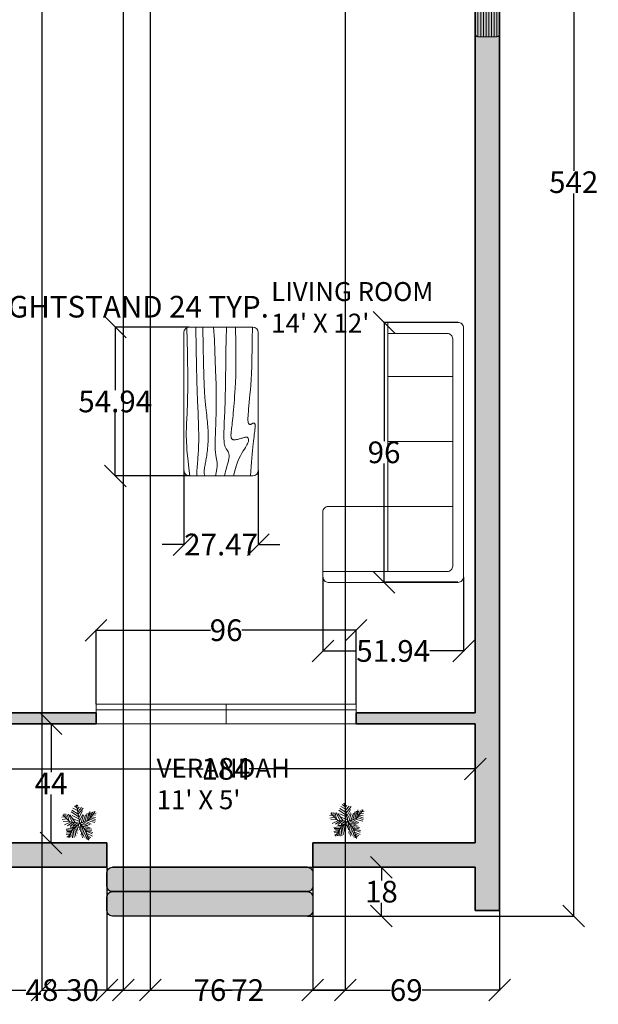
# Model space of a CAD drawing. Units: inches. Extents: x -8 to 447, y -560 to 47.
# Tile 2 of 5: x 201 to 415, y -560 to -196. Entities that reach past the tile are written whole.
import ezdxf

# ---------------------------------------------------------------- set-up
doc = ezdxf.new("R2010")
doc.units = ezdxf.units.IN
doc.header["$MEASUREMENT"] = 0
for name, color, linetype, lineweight in [('A-ANNO-DIMS', 2, 'Continuous', 18), ('A-AREA-IDEN', 7, 'Continuous', 18), ('A-FLOR-PATT', 251, 'Continuous', 13), ('A-FLOR-STRS', 7, 'Continuous', 25), ('A-FURN', 8, 'Continuous', 18), ('A-WALL', 7, 'Continuous', 35), ('A-WALL-PATT', 251, 'Continuous', 13), ('DOOR', 40, 'Continuous', 18), ('PLANTS', 82, 'Continuous', 13), ('WINDOW', 151, 'Continuous', 13)]:
    doc.layers.add(name, color=color, linetype=linetype, lineweight=lineweight)
doc.styles.get("Standard").update_dxf_attribs({"font": 'arial.ttf'})
doc.dimstyles.get("Standard").update_dxf_attribs({"dimtxt": 8, "dimasz": 8, "dimexe": 0.18, "dimexo": 0.0625, "dimgap": 0.09, "dimtad": 0, "dimtih": 1, "dimtoh": 1, "dimdec": 0, "dimzin": 0, "dimdsep": 46, "dimlunit": 4, "dimtxsty": 'Standard', "dimblk": 'OBLIQUE', "dimcen": 0.09, "dimadec": 0, "dimazin": 0, "dimtfac": 1, "dimtdec": 0, "dimtofl": 0, "dimtmove": 0, "dimatfit": 3, "dimldrblk": 'OBLIQUE', "dimfxl": 1, "dimtolj": 1, "dimtzin": 0, "dimarcsym": 0})

# ---------------------------------------------------------------- blocks, each defined once
blk = doc.blocks.new('WINDOW')
for p, q in [((0, -1.63), (48, -1.63)), ((0, -2.63), (48, -2.63)), ((0, -3.63), (48, -3.63)), ((0, -4.63), (48, -4.63)), ((0, -5.63), (48, -5.63)), ((0, -6.63), (48, -6.63)), ((0, -7.63), (48, -7.63)), ((0, -8.63), (48, -8.63))]:
    blk.add_line(p, q)
blk.add_lwpolyline([(48, -1.63), (48, -8.63, -0.414214), (47, -9.63), (1, -9.63, -0.414214), (0, -8.63), (0, -1.63, -0.414214), (1, -0.63), (47, -0.63, -0.414214)], format="xyb", close=True)
blk = doc.blocks.new('*U7')
for p, q in [((0, 0), (0, -6)), ((40, 0), (40, -6))]:
    blk.add_line(p, q)
blk.add_lwpolyline([(0, 0), (40, 0), (40, -1.75), (0, -1.75)], close=True)
blk = doc.blocks.new('*U23')
for p, q in [((-3.665, 19.273), (-27.574, 35.527)), ((-5.114, 28.097), (-24.676, 40.636)), ((-7.288, 39.707), (-21.778, 46.673)), ((-8.737, 47.138), (-17.069, 52.711)), ((-10.186, 53.64), (-13.084, 55.962)), ((0, 0), (-10.5, 57)), ((-9.099, 51.782), (-6.563, 55.962)), ((-7.65, 43.423), (-2.578, 49.46)), ((-5.839, 35.992), (4.667, 48.067)), ((-5.114, 27.632), (10.463, 46.673)), ((-2.941, 16.486), (8.652, 37.85)), ((16.259, 5.805), (23.142, 31.348)), ((22.055, 7.198), (27.489, 32.277)), ((27, 9), (48, 36)), ((27.127, 9.056), (31.112, 35.992)), ((31.836, 30.883), (32.561, 16.486)), ((35.096, 32.741), (37.27, 22.524)), ((38.719, 34.134), (41.979, 28.561)), ((43.791, 29.954), (51.036, 30.883)), ((44.153, 36.456), (45.239, 32.741)), ((-47.498, 19.737), (-55.83, 18.344)), ((-40.615, 13.7), (-55.105, 10.913)), ((-31.5, 4.5), (-52.5, 25.5)), ((-33.37, 6.269), (-52.207, 5.34)), ((-48.585, 21.131), (-49.309, 29.026)), ((-28.299, 3.483), (-47.86, -5.805)), ((-43.513, 28.561), (-42.427, 15.558)), ((-38.442, 26.239), (-34.819, 7.663)), ((-21.416, 3.018), (-38.079, -8.128)), ((-35.544, 28.097), (-24.314, 3.947)), ((0, 0), (-31.5, 4.5)), ((-14.533, 2.09), (-30.834, 25.31)), ((-15.982, 2.09), (-30.11, -9.521)), ((-24.314, 23.917), (-2.941, 13.7)), ((0, 0), (-22.5, -19.5)), ((-6.563, 1.161), (-21.416, -8.128)), ((-20.691, 13.7), (-1.129, 4.876)), ((-1.129, 6.734), (9.014, 26.704)), ((0, 0), (27, 9)), ((0, 0), (18, -22.5)), ((3.942, 1.625), (11.187, 24.381)), ((6.478, 1.625), (26.04, -8.592)), ((10.101, 3.483), (17.708, 26.239)), ((11.187, 3.483), (30.749, -5.805)), ((18.07, 5.805), (35.096, -3.483)), ((24.229, 7.663), (46.688, 1.625)), ((29.662, 12.307), (48.137, 6.269)), ((33.285, 16.486), (48.862, 10.913)), ((36.183, 19.737), (48.137, 17.88)), ((40.53, 25.775), (48.862, 24.846)), ((-17.431, -15.094), (-42.789, -18.809)), ((-28.299, -29.026), (-42.789, -31.348)), ((-24.314, -21.596), (-42.427, -22.06)), ((-26.849, -26.24), (-40.253, -25.775)), ((-22.5, -19.5), (-37.5, -45)), ((-15.257, -12.772), (-30.11, -12.772)), ((-25.038, -23.918), (-22.865, -45.281)), ((-20.691, -18.345), (-17.793, -44.352)), ((-6.563, -5.805), (-19.967, -9.985)), ((-17.069, -15.094), (-12.721, -40.172)), ((-13.446, -11.378), (-8.737, -32.741)), ((-9.461, -8.592), (-6.201, -23.453)), ((-4.752, -3.483), (-3.665, -14.629)), ((2.493, -3.019), (-1.491, -20.202)), ((1.769, -2.555), (24.229, -9.521)), ((5.029, -6.27), (2.131, -25.775)), ((9.014, -11.378), (3.58, -35.992)), ((14.085, -16.951), (6.478, -40.172)), ((7.565, -9.056), (32.198, -14.629)), ((18.07, -22.524), (8.289, -45.745)), ((12.274, -15.094), (36.907, -18.809)), ((20.244, -30.419), (15.897, -44.816)), ((16.259, -19.738), (36.183, -22.989)), ((18, -22.5), (27, -52.5)), ((18.433, -22.524), (40.53, -29.026)), ((19.157, -25.311), (38.719, -33.206)), ((-30.834, -34.135), (-42.427, -35.528)), ((-34.457, -39.708), (-40.978, -42.494)), ((-32.646, -36.921), (-31.921, -44.352)), ((-29.023, -30.884), (-27.936, -43.887)), ((22.78, -37.85), (19.519, -48.532)), ((21.331, -32.741), (39.081, -40.636)), ((22.78, -38.314), (34.372, -44.816)), ((24.591, -45.745), (23.142, -50.854)), ((24.591, -43.423), (30.749, -47.603)), ((26.764, -49.925), (28.213, -50.854))]:
    blk.add_line(p, q)
blk = doc.blocks.new('_Oblique')
at = {"color": 0, "linetype": 'ByBlock', "lineweight": -2}
blk.add_line((-0.5, -0.5), (0.5, 0.5), dxfattribs=at)
blk = doc.blocks.new('*D33')
at = {"layer": 'A-ANNO-DIMS', "color": 0, "lineweight": -2, "transparency": 16777216}
for p, q in [((150.53, -305.97), (150.53, -302.25)), ((150.53, -302.43), (174.53, -302.43)), ((174.53, -305.97), (174.53, -302.25)), ((174.53, -302.43), (182.53, -302.43))]:
    blk.add_line(p, q, dxfattribs=at)
at = {"layer": 'Defpoints', "color": 0, "transparency": 16777216}
for p in [(174.53, -302.43), (150.53, -306.03), (174.53, -306.03)]:
    blk.add_point(p, dxfattribs=at)
at = {"layer": 'A-ANNO-DIMS', "color": 0, "lineweight": -2, "transparency": 16777216, "xscale": 8, "yscale": 8, "zscale": 8, "rotation": 180}
blk.add_blockref('_Oblique', (150.53, -302.43), dxfattribs=at)
at = {"layer": 'A-ANNO-DIMS', "color": 0, "lineweight": -2, "transparency": 16777216, "xscale": 8, "yscale": 8, "zscale": 8}
blk.add_blockref('_Oblique', (174.53, -302.43), dxfattribs=at)
at = {"layer": 'A-ANNO-DIMS', "color": 0, "transparency": 16777216, "insert": (239.77, -302.43), "char_height": 8, "attachment_point": 5}
blk.add_mtext('\\A1;NIGHTSTAND 24 TYP.', dxfattribs=at)
blk = doc.blocks.new('*D52')
at = {"layer": 'A-ANNO-DIMS', "color": 0, "lineweight": -2, "transparency": 16777216}
for p, q in [((378.76, 14.56), (406.23, 14.56)), ((406.05, 14.56), (406.05, -252.27)), ((406.05, -527.44), (406.05, -260.61)), ((307.76, -527.44), (406.23, -527.44))]:
    blk.add_line(p, q, dxfattribs=at)
at = {"layer": 'Defpoints', "color": 0, "transparency": 16777216}
for p in [(378.7, 14.56), (307.7, -527.44), (406.05, -527.44)]:
    blk.add_point(p, dxfattribs=at)
at = {"layer": 'A-ANNO-DIMS', "color": 0, "lineweight": -2, "transparency": 16777216, "xscale": 8, "yscale": 8, "zscale": 8}
for p, rotation in [((406.05, 14.56), 90), ((406.05, -527.44), 270)]:
    blk.add_blockref('_Oblique', p, dxfattribs=dict(at, rotation=rotation))
at = {"layer": 'A-ANNO-DIMS', "color": 0, "transparency": 16777216, "insert": (406.05, -256.44), "char_height": 8, "attachment_point": 5}
blk.add_mtext('\\A1;542', dxfattribs=at)
blk = doc.blocks.new('*D59')
at = {"layer": 'A-ANNO-DIMS', "color": 0, "lineweight": -2, "transparency": 16777216}
for p, q in [((233.7, -509.5), (233.7, -554.97)), ((185.7, -525.5), (185.7, -554.97)), ((185.7, -554.79), (203.71, -554.79)), ((233.7, -554.79), (215.69, -554.79))]:
    blk.add_line(p, q, dxfattribs=at)
at = {"layer": 'Defpoints', "color": 0, "transparency": 16777216}
for p in [(233.7, -509.44), (185.7, -525.44), (233.7, -554.79)]:
    blk.add_point(p, dxfattribs=at)
at = {"layer": 'A-ANNO-DIMS', "color": 0, "lineweight": -2, "transparency": 16777216, "xscale": 8, "yscale": 8, "zscale": 8, "rotation": 180}
blk.add_blockref('_Oblique', (185.7, -554.79), dxfattribs=at)
at = {"layer": 'A-ANNO-DIMS', "color": 0, "lineweight": -2, "transparency": 16777216, "xscale": 8, "yscale": 8, "zscale": 8}
blk.add_blockref('_Oblique', (233.7, -554.79), dxfattribs=at)
at = {"layer": 'A-ANNO-DIMS', "color": 0, "transparency": 16777216, "insert": (209.7, -554.79), "char_height": 8, "attachment_point": 5}
blk.add_mtext('\\A1;48', dxfattribs=at)
blk = doc.blocks.new('*D60')
at = {"layer": 'A-ANNO-DIMS', "color": 0, "lineweight": -2, "transparency": 16777216}
for p, q in [((233.7, -509.5), (233.7, -554.97)), ((309.7, -509.5), (309.7, -554.97)), ((233.7, -554.79), (265.92, -554.79)), ((309.7, -554.79), (277.49, -554.79))]:
    blk.add_line(p, q, dxfattribs=at)
at = {"layer": 'Defpoints', "color": 0, "transparency": 16777216}
for p in [(233.7, -509.44), (309.7, -509.44), (309.7, -554.79)]:
    blk.add_point(p, dxfattribs=at)
at = {"layer": 'A-ANNO-DIMS', "color": 0, "lineweight": -2, "transparency": 16777216, "xscale": 8, "yscale": 8, "zscale": 8, "rotation": 180}
blk.add_blockref('_Oblique', (233.7, -554.79), dxfattribs=at)
at = {"layer": 'A-ANNO-DIMS', "color": 0, "lineweight": -2, "transparency": 16777216, "xscale": 8, "yscale": 8, "zscale": 8}
blk.add_blockref('_Oblique', (309.7, -554.79), dxfattribs=at)
at = {"layer": 'A-ANNO-DIMS', "color": 0, "transparency": 16777216, "insert": (271.7, -554.79), "char_height": 8, "attachment_point": 5}
blk.add_mtext('\\A1;76', dxfattribs=at)
blk = doc.blocks.new('*D61')
at = {"layer": 'A-ANNO-DIMS', "color": 0, "lineweight": -2, "transparency": 16777216}
for p, q in [((309.7, -509.5), (309.7, -554.97)), ((378.7, -525.5), (378.7, -554.97)), ((309.7, -554.79), (338.35, -554.79)), ((378.7, -554.79), (350.05, -554.79))]:
    blk.add_line(p, q, dxfattribs=at)
at = {"layer": 'Defpoints', "color": 0, "transparency": 16777216}
for p in [(309.7, -509.44), (378.7, -525.44), (378.7, -554.79)]:
    blk.add_point(p, dxfattribs=at)
at = {"layer": 'A-ANNO-DIMS', "color": 0, "lineweight": -2, "transparency": 16777216, "xscale": 8, "yscale": 8, "zscale": 8, "rotation": 180}
blk.add_blockref('_Oblique', (309.7, -554.79), dxfattribs=at)
at = {"layer": 'A-ANNO-DIMS', "color": 0, "lineweight": -2, "transparency": 16777216, "xscale": 8, "yscale": 8, "zscale": 8}
blk.add_blockref('_Oblique', (378.7, -554.79), dxfattribs=at)
at = {"layer": 'A-ANNO-DIMS', "color": 0, "transparency": 16777216, "insert": (344.2, -554.79), "char_height": 8, "attachment_point": 5}
blk.add_mtext('\\A1;69', dxfattribs=at)
blk = doc.blocks.new('*D62')
at = {"layer": 'A-ANNO-DIMS', "color": 0, "lineweight": -2, "transparency": 16777216}
for p, q in [((209.7, -94.5), (209.7, -554.97)), ((239.7, -94.5), (239.7, -554.97)), ((209.7, -554.79), (218.9, -554.79)), ((239.7, -554.79), (230.51, -554.79))]:
    blk.add_line(p, q, dxfattribs=at)
at = {"layer": 'Defpoints', "color": 0, "transparency": 16777216}
for p in [(209.7, -94.44), (239.7, -94.44), (239.7, -554.79)]:
    blk.add_point(p, dxfattribs=at)
at = {"layer": 'A-ANNO-DIMS', "color": 0, "lineweight": -2, "transparency": 16777216, "xscale": 8, "yscale": 8, "zscale": 8, "rotation": 180}
blk.add_blockref('_Oblique', (209.7, -554.79), dxfattribs=at)
at = {"layer": 'A-ANNO-DIMS', "color": 0, "lineweight": -2, "transparency": 16777216, "xscale": 8, "yscale": 8, "zscale": 8}
blk.add_blockref('_Oblique', (239.7, -554.79), dxfattribs=at)
at = {"layer": 'A-ANNO-DIMS', "color": 0, "transparency": 16777216, "insert": (224.7, -554.79), "char_height": 8, "attachment_point": 5}
blk.add_mtext('\\A1;30', dxfattribs=at)
blk = doc.blocks.new('*D63')
at = {"layer": 'A-ANNO-DIMS', "color": 0, "lineweight": -2, "transparency": 16777216}
for p, q in [((249.7, -94.5), (249.7, -554.97)), ((321.7, -94.5), (321.7, -554.97)), ((249.7, -554.79), (279.96, -554.79)), ((321.7, -554.79), (291.45, -554.79))]:
    blk.add_line(p, q, dxfattribs=at)
at = {"layer": 'Defpoints', "color": 0, "transparency": 16777216}
for p in [(249.7, -94.44), (321.7, -94.44), (321.7, -554.79)]:
    blk.add_point(p, dxfattribs=at)
at = {"layer": 'A-ANNO-DIMS', "color": 0, "lineweight": -2, "transparency": 16777216, "xscale": 8, "yscale": 8, "zscale": 8, "rotation": 180}
blk.add_blockref('_Oblique', (249.7, -554.79), dxfattribs=at)
at = {"layer": 'A-ANNO-DIMS', "color": 0, "lineweight": -2, "transparency": 16777216, "xscale": 8, "yscale": 8, "zscale": 8}
blk.add_blockref('_Oblique', (321.7, -554.79), dxfattribs=at)
at = {"layer": 'A-ANNO-DIMS', "color": 0, "transparency": 16777216, "insert": (285.7, -554.79), "char_height": 8, "attachment_point": 5}
blk.add_mtext('\\A1;72', dxfattribs=at)
blk = doc.blocks.new('*D64')
at = {"layer": 'A-ANNO-DIMS', "color": 0, "lineweight": -2, "transparency": 16777216}
for p, q in [((185.7, -500.38), (185.7, -472.91)), ((185.7, -473.09), (269.17, -473.09)), ((369.7, -473.09), (286.24, -473.09)), ((369.7, -500.38), (369.7, -472.91))]:
    blk.add_line(p, q, dxfattribs=at)
at = {"layer": 'Defpoints', "color": 0, "transparency": 16777216}
for p in [(369.7, -473.09), (185.7, -500.44), (369.7, -500.44)]:
    blk.add_point(p, dxfattribs=at)
at = {"layer": 'A-ANNO-DIMS', "color": 0, "lineweight": -2, "transparency": 16777216, "xscale": 8, "yscale": 8, "zscale": 8, "rotation": 180}
blk.add_blockref('_Oblique', (185.7, -473.09), dxfattribs=at)
at = {"layer": 'A-ANNO-DIMS', "color": 0, "lineweight": -2, "transparency": 16777216, "xscale": 8, "yscale": 8, "zscale": 8}
blk.add_blockref('_Oblique', (369.7, -473.09), dxfattribs=at)
at = {"layer": 'A-ANNO-DIMS', "color": 0, "transparency": 16777216, "insert": (277.7, -473.09), "char_height": 8, "attachment_point": 5}
blk.add_mtext('\\A1;184', dxfattribs=at)
blk = doc.blocks.new('*D65')
at = {"layer": 'A-ANNO-DIMS', "color": 0, "lineweight": -2, "transparency": 16777216}
for p, q in [((185.764836, -456.440047), (213.232336, -456.440047)), ((213.052336, -456.440047), (213.052336, -474.350047)), ((213.052336, -500.440047), (213.052336, -482.530047)), ((185.764836, -500.440047), (213.232336, -500.440047))]:
    blk.add_line(p, q, dxfattribs=at)
at = {"layer": 'Defpoints', "color": 0, "transparency": 16777216}
for p in [(185.702336, -456.440047), (185.702336, -500.440047), (213.052336, -500.440047)]:
    blk.add_point(p, dxfattribs=at)
at = {"layer": 'A-ANNO-DIMS', "color": 0, "lineweight": -2, "transparency": 16777216, "xscale": 8, "yscale": 8, "zscale": 8}
for p, rotation in [((213.052336, -456.440047), 90), ((213.052336, -500.440047), 270)]:
    blk.add_blockref('_Oblique', p, dxfattribs=dict(at, rotation=rotation))
at = {"layer": 'A-ANNO-DIMS', "color": 0, "transparency": 16777216, "insert": (213.052336, -478.440047), "char_height": 8, "attachment_point": 5}
blk.add_mtext('\\A1;44', dxfattribs=at)
blk = doc.blocks.new('*D70')
at = {"layer": 'A-ANNO-DIMS', "color": 0, "lineweight": -2, "transparency": 16777216}
for p, q in [((229.7, -449.18), (229.7, -421.71)), ((325.7, -449.18), (325.7, -421.71)), ((229.7, -421.89), (271.89, -421.89)), ((325.7, -421.89), (283.52, -421.89))]:
    blk.add_line(p, q, dxfattribs=at)
at = {"layer": 'Defpoints', "color": 0, "transparency": 16777216}
for p in [(325.7, -421.89), (229.7, -449.24), (325.7, -449.24)]:
    blk.add_point(p, dxfattribs=at)
at = {"layer": 'A-ANNO-DIMS', "color": 0, "lineweight": -2, "transparency": 16777216, "xscale": 8, "yscale": 8, "zscale": 8, "rotation": 180}
blk.add_blockref('_Oblique', (229.7, -421.89), dxfattribs=at)
at = {"layer": 'A-ANNO-DIMS', "color": 0, "lineweight": -2, "transparency": 16777216, "xscale": 8, "yscale": 8, "zscale": 8}
blk.add_blockref('_Oblique', (325.7, -421.89), dxfattribs=at)
at = {"layer": 'A-ANNO-DIMS', "color": 0, "transparency": 16777216, "insert": (277.7, -421.89), "char_height": 8, "attachment_point": 5}
blk.add_mtext('\\A1;96', dxfattribs=at)
blk = doc.blocks.new('*D71')
at = {"layer": 'A-ANNO-DIMS', "color": 0, "lineweight": -2, "transparency": 16777216}
for p, q in [((307.76, -509.44), (335.23, -509.44)), ((335.05, -509.44), (335.05, -514.27)), ((335.05, -527.44), (335.05, -522.61)), ((307.76, -527.44), (335.23, -527.44))]:
    blk.add_line(p, q, dxfattribs=at)
at = {"layer": 'Defpoints', "color": 0, "transparency": 16777216}
for p in [(307.7, -509.44), (307.7, -527.44), (335.05, -527.44)]:
    blk.add_point(p, dxfattribs=at)
at = {"layer": 'A-ANNO-DIMS', "color": 0, "lineweight": -2, "transparency": 16777216, "xscale": 8, "yscale": 8, "zscale": 8}
for p, rotation in [((335.05, -509.44), 90), ((335.05, -527.44), 270)]:
    blk.add_blockref('_Oblique', p, dxfattribs=dict(at, rotation=rotation))
at = {"layer": 'A-ANNO-DIMS', "color": 0, "transparency": 16777216, "insert": (335.05, -518.44), "char_height": 8, "attachment_point": 5}
blk.add_mtext('\\A1;18', dxfattribs=at)
blk = doc.blocks.new('*D72')
at = {"layer": 'A-ANNO-DIMS', "color": 0, "lineweight": -2, "transparency": 16777216}
for p, q in [((313.43, -402.28), (313.43, -429.74)), ((365.37, -402.28), (365.37, -429.74)), ((313.43, -429.56), (325.83, -429.56)), ((365.37, -429.56), (352.97, -429.56))]:
    blk.add_line(p, q, dxfattribs=at)
at = {"layer": 'Defpoints', "color": 0, "transparency": 16777216}
for p in [(313.43, -402.21), (365.37, -402.21), (313.43, -429.56)]:
    blk.add_point(p, dxfattribs=at)
at = {"layer": 'A-ANNO-DIMS', "color": 0, "lineweight": -2, "transparency": 16777216, "xscale": 8, "yscale": 8, "zscale": 8, "rotation": 180}
blk.add_blockref('_Oblique', (313.43, -429.56), dxfattribs=at)
at = {"layer": 'A-ANNO-DIMS', "color": 0, "lineweight": -2, "transparency": 16777216, "xscale": 8, "yscale": 8, "zscale": 8}
blk.add_blockref('_Oblique', (365.37, -429.56), dxfattribs=at)
at = {"layer": 'A-ANNO-DIMS', "color": 0, "transparency": 16777216, "insert": (339.4, -429.56), "char_height": 8, "attachment_point": 5}
blk.add_mtext('\\A1;51.94', dxfattribs=at)
blk = doc.blocks.new('*D73')
at = {"layer": 'A-ANNO-DIMS', "color": 0, "lineweight": -2, "transparency": 16777216}
for p, q in [((363.31, -308.21), (335.84, -308.21)), ((336.02, -308.21), (336.02, -352.04)), ((336.02, -404.21), (336.02, -360.39)), ((363.31, -404.21), (335.84, -404.21))]:
    blk.add_line(p, q, dxfattribs=at)
at = {"layer": 'Defpoints', "color": 0, "transparency": 16777216}
for p in [(336.02, -308.21), (363.37, -308.21), (363.37, -404.21)]:
    blk.add_point(p, dxfattribs=at)
at = {"layer": 'A-ANNO-DIMS', "color": 0, "lineweight": -2, "transparency": 16777216, "xscale": 8, "yscale": 8, "zscale": 8}
for p, rotation in [((336.02, -308.21), 90), ((336.02, -404.21), 270)]:
    blk.add_blockref('_Oblique', p, dxfattribs=dict(at, rotation=rotation))
at = {"layer": 'A-ANNO-DIMS', "color": 0, "transparency": 16777216, "insert": (336.02, -356.21), "char_height": 8, "attachment_point": 5}
blk.add_mtext('\\A1;96', dxfattribs=at)
blk = doc.blocks.new('*D74')
at = {"layer": 'A-ANNO-DIMS', "color": 0, "lineweight": -2, "transparency": 16777216}
for p, q in [((262.111265, -362.959517), (262.111265, -390.427017)), ((289.583453, -362.959517), (289.583453, -390.427017)), ((262.111265, -390.247017), (254.111265, -390.247017)), ((289.583453, -390.247017), (297.583453, -390.247017))]:
    blk.add_line(p, q, dxfattribs=at)
at = {"layer": 'Defpoints', "color": 0, "transparency": 16777216}
for p in [(262.111265, -362.897017), (289.583453, -362.897017), (262.111265, -390.247017)]:
    blk.add_point(p, dxfattribs=at)
at = {"layer": 'A-ANNO-DIMS', "color": 0, "lineweight": -2, "transparency": 16777216, "xscale": 8, "yscale": 8, "zscale": 8}
blk.add_blockref('_Oblique', (262.111265, -390.247017), dxfattribs=at)
at = {"layer": 'A-ANNO-DIMS', "color": 0, "lineweight": -2, "transparency": 16777216, "xscale": 8, "yscale": 8, "zscale": 8, "rotation": 180}
blk.add_blockref('_Oblique', (289.583453, -390.247017), dxfattribs=at)
at = {"layer": 'A-ANNO-DIMS', "color": 0, "transparency": 16777216, "insert": (275.847359, -390.247017), "char_height": 8, "attachment_point": 5}
blk.add_mtext('\\A1;27.47', dxfattribs=at)
blk = doc.blocks.new('*D75')
at = {"layer": 'A-ANNO-DIMS', "color": 0, "lineweight": -2, "transparency": 16777216}
for p, q in [((264.05, -309.95), (236.58, -309.95)), ((236.76, -309.95), (236.76, -333.25)), ((236.76, -364.9), (236.76, -341.6)), ((264.05, -364.9), (236.58, -364.9))]:
    blk.add_line(p, q, dxfattribs=at)
at = {"layer": 'Defpoints', "color": 0, "transparency": 16777216}
for p in [(236.76, -309.95), (264.11, -309.95), (264.11, -364.9)]:
    blk.add_point(p, dxfattribs=at)
at = {"layer": 'A-ANNO-DIMS', "color": 0, "lineweight": -2, "transparency": 16777216, "xscale": 8, "yscale": 8, "zscale": 8}
for p, rotation in [((236.76, -309.95), 90), ((236.76, -364.9), 270)]:
    blk.add_blockref('_Oblique', p, dxfattribs=dict(at, rotation=rotation))
at = {"layer": 'A-ANNO-DIMS', "color": 0, "transparency": 16777216, "insert": (236.76, -337.42), "char_height": 8, "attachment_point": 5}
blk.add_mtext('\\A1;54.94', dxfattribs=at)

msp = doc.modelspace()

# ---------------------------------------------------------------- hatches: boundary and pattern name
at = {"layer": 'A-FLOR-PATT'}
h = msp.add_hatch(color=256, dxfattribs=at)
h.dxf.hatch_style = 1
h.paths.add_polyline_path([(309.702, -511.44, 0.4142136), (307.702, -509.44), (235.702, -509.44, 0.4142136), (233.702, -511.44), (233.702, -516.44, 0.4142136), (235.702, -518.44), (307.702, -518.44, 0.4142136), (309.702, -516.44)])
h.paths.add_polyline_path([(309.702, -520.44, 0.4142136), (307.702, -518.44), (235.702, -518.44, 0.4142136), (233.702, -520.44), (233.702, -525.44, 0.4142136), (235.702, -527.44), (307.702, -527.44, 0.4142136), (309.702, -525.44)])
at = {"layer": 'A-WALL-PATT'}
h = msp.add_hatch(color=256, dxfattribs=at)
h.dxf.hatch_style = 1
h.paths.add_polyline_path([(378.702, 14.56), (227.702, 14.56), (227.702, 5.56), (245.702, 5.56), (245.702, -90.44), (239.702, -90.44), (239.702, -94.44), (249.702, -94.44), (249.702, -90.44), (249.702, 5.56), (369.702, 5.56), (369.702, -90.44), (321.702, -90.44), (321.702, -94.44), (369.702, -94.44), (369.702, -452.44), (325.702, -452.44), (325.702, -456.44), (369.702, -456.44), (369.702, -500.44), (309.702, -500.44), (309.702, -509.44), (369.702, -509.44), (369.702, -525.44), (378.702, -525.44)])
h = msp.add_hatch(color=256, dxfattribs=at)
h.dxf.hatch_style = 1
h.paths.add_polyline_path([(61.702, -516.44), (37.702, -516.44), (37.702, -435.116), (28.702, -435.116), (28.702, -525.44), (61.702, -525.44)])
h.paths.add_polyline_path([(185.702, -509.44), (233.702, -509.44), (233.702, -500.44), (185.702, -500.44), (185.702, -492.44), (181.702, -492.44), (181.702, -516.44), (157.702, -516.44), (157.702, -525.44), (185.702, -525.44)])
h.paths.add_polyline_path([(229.702, -452.44), (185.702, -452.44), (185.702, -428.44), (181.702, -428.44), (181.702, -462.44), (185.702, -462.44), (185.702, -456.44), (229.702, -456.44)])

# ---------------------------------------------------------------- linework, layer by layer
at = {"layer": 'A-FLOR-STRS'}
for points in [[(233.702, -509.44), (233.702, -500.44)], [(309.702, -500.44), (309.702, -509.44)], [(307.702, -509.44), (235.702, -509.44)]]:
    msp.add_lwpolyline(points, dxfattribs=at)
for points in [[(235.702, -509.44), (307.702, -509.44, -0.4142136), (309.702, -511.44), (309.702, -516.44, -0.4142136), (307.702, -518.44), (235.702, -518.44, -0.4142136), (233.702, -516.44), (233.702, -511.44, -0.4142136)], [(235.702, -518.44), (307.702, -518.44, -0.4142136), (309.702, -520.44), (309.702, -525.44, -0.4142136), (307.702, -527.44), (235.702, -527.44, -0.4142136), (233.702, -525.44), (233.702, -520.44, -0.4142136)]]:
    msp.add_lwpolyline(points, format="xyb", close=True, dxfattribs=at)
at = {"layer": 'A-FURN'}
for p, q in [((262.111, -311.953), (262.111, -362.897)), ((287.583, -309.953), (264.111, -309.953)), ((289.583, -362.897), (289.583, -311.953)), ((264.111, -364.897), (287.583, -364.897))]:
    msp.add_line(p, q, dxfattribs=at)
for points in [[(337.369, -312.214), (337.369, -308.214), (361.369, -308.214), (363.369, -308.214, -0.4142136), (365.369, -310.214), (365.369, -402.214, -0.4142136), (363.369, -404.214), (361.369, -404.214), (315.429, -404.214, -0.4142136), (313.429, -402.214), (313.429, -378.214, -0.4142136), (315.429, -376.214), (337.429, -376.214), (361.369, -376.214), (361.369, -398.214)], [(337.429, -336.305), (337.429, -312.305), (359.369, -312.305, -0.4142136), (361.369, -314.305), (361.369, -336.305)], [(313.429, -400.214), (337.369, -400.214), (359.369, -400.214, 0.4142136), (361.369, -398.214), (361.369, -314.305)]]:
    msp.add_lwpolyline(points, format="xyb", dxfattribs=at)
for points in [[(263.215, -310.165), (263.331, -315.16), (263.421, -319.522), (263.484, -323.146), (263.523, -326.138), (263.542, -328.607), (263.545, -330.66), (263.535, -332.403), (263.515, -333.945), (263.49, -335.375), (263.459, -336.718), (263.424, -337.977), (263.386, -339.161), (263.344, -340.274), (263.301, -341.324), (263.256, -342.315), (263.21, -343.255), (263.165, -344.15), (263.121, -345.014), (263.081, -345.862), (263.046, -346.708), (263.018, -347.567), (263, -348.453), (262.992, -349.382), (262.997, -350.367), (263.017, -351.43), (263.06, -352.612), (263.135, -353.961), (263.252, -355.526), (263.419, -357.354), (263.645, -359.493), (263.938, -361.992), (264.309, -364.897)], [(266.507, -309.953), (266.644, -317.861), (266.779, -324.332), (266.909, -329.554), (267.033, -333.712), (267.149, -336.994), (267.254, -339.584), (267.346, -341.67), (267.423, -343.438), (267.483, -345.045), (267.527, -346.529), (267.558, -347.898), (267.575, -349.162), (267.581, -350.328), (267.577, -351.405), (267.564, -352.402), (267.545, -353.328), (267.519, -354.191), (267.488, -355), (267.452, -355.766), (267.411, -356.496), (267.366, -357.201), (267.317, -357.89), (267.265, -358.572), (267.209, -359.258), (267.151, -359.953), (267.092, -360.657), (267.036, -361.367), (266.984, -362.08), (266.939, -362.793), (266.904, -363.502), (266.881, -364.204), (266.873, -364.897)], [(269.071, -309.953), (269.208, -317.288), (269.345, -323.148), (269.48, -327.733), (269.613, -331.244), (269.743, -333.878), (269.869, -335.837), (269.991, -337.319), (270.109, -338.524), (270.22, -339.62), (270.326, -340.646), (270.426, -341.609), (270.521, -342.519), (270.61, -343.381), (270.692, -344.203), (270.77, -344.993), (270.841, -345.758), (270.907, -346.506), (270.965, -347.24), (271.015, -347.967), (271.055, -348.688), (271.083, -349.41), (271.099, -350.136), (271.1, -350.871), (271.086, -351.619), (271.054, -352.381), (271.008, -353.152), (270.949, -353.923), (270.879, -354.685), (270.801, -355.428), (270.716, -356.145), (270.627, -356.827), (270.536, -357.464), (270.445, -358.051), (270.353, -358.594), (270.263, -359.099), (270.174, -359.574), (270.086, -360.028), (270, -360.469), (269.915, -360.904), (269.834, -361.341), (269.756, -361.786), (269.688, -362.238), (269.634, -362.693), (269.601, -363.148), (269.596, -363.599), (269.624, -364.043), (269.691, -364.477), (269.803, -364.897)], [(273.1, -309.953), (273.35, -314.645), (273.553, -318.8), (273.713, -322.471), (273.837, -325.715), (273.927, -328.585), (273.989, -331.136), (274.027, -333.424), (274.046, -335.502), (274.051, -337.418), (274.043, -339.192), (274.024, -340.836), (273.997, -342.362), (273.962, -343.782), (273.922, -345.108), (273.878, -346.353), (273.833, -347.528), (273.787, -348.644), (273.744, -349.702), (273.705, -350.702), (273.672, -351.642), (273.648, -352.522), (273.635, -353.341), (273.635, -354.098), (273.65, -354.793), (273.681, -355.427), (273.726, -356.003), (273.783, -356.527), (273.848, -357.004), (273.919, -357.441), (273.993, -357.843), (274.067, -358.215), (274.138, -358.563), (274.204, -358.893), (274.262, -359.209), (274.312, -359.52), (274.352, -359.83), (274.38, -360.146), (274.396, -360.473), (274.397, -360.819), (274.382, -361.188), (274.351, -361.585), (274.307, -361.998), (274.252, -362.417), (274.191, -362.827), (274.128, -363.217), (274.065, -363.573), (274.006, -363.883), (273.955, -364.134), (273.915, -364.318), (273.884, -364.446), (273.862, -364.534), (273.848, -364.596), (273.839, -364.647), (273.835, -364.705), (273.833, -364.783), (273.833, -364.897)], [(277.862, -309.953), (277.741, -314.7), (277.649, -318.763), (277.582, -322.22), (277.534, -325.15), (277.5, -327.632), (277.476, -329.745), (277.455, -331.569), (277.435, -333.182), (277.409, -334.653), (277.378, -336.008), (277.343, -337.265), (277.305, -338.44), (277.264, -339.549), (277.22, -340.608), (277.175, -341.634), (277.129, -342.645), (277.084, -343.65), (277.04, -344.648), (276.998, -345.628), (276.962, -346.582), (276.93, -347.502), (276.906, -348.379), (276.891, -349.205), (276.885, -349.97), (276.891, -350.669), (276.908, -351.303), (276.937, -351.875), (276.977, -352.389), (277.028, -352.849), (277.091, -353.259), (277.166, -353.62), (277.251, -353.939), (277.348, -354.217), (277.455, -354.461), (277.568, -354.677), (277.686, -354.87), (277.808, -355.045), (277.93, -355.209), (278.05, -355.368), (278.167, -355.526), (278.279, -355.689), (278.383, -355.861), (278.478, -356.042), (278.564, -356.236), (278.638, -356.443), (278.7, -356.668), (278.746, -356.911), (278.778, -357.174), (278.792, -357.46), (278.79, -357.765), (278.772, -358.086), (278.74, -358.419), (278.692, -358.761), (278.632, -359.109), (278.558, -359.459), (278.473, -359.807), (278.375, -360.156), (278.263, -360.528), (278.133, -360.954), (277.984, -361.462), (277.812, -362.081), (277.614, -362.841), (277.387, -363.77), (277.129, -364.897)], [(281.159, -309.953), (281.263, -315.974), (281.308, -320.885), (281.304, -324.836), (281.258, -327.977), (281.181, -330.461), (281.081, -332.437), (280.969, -334.057), (280.853, -335.471), (280.742, -336.806), (280.635, -338.084), (280.533, -339.305), (280.434, -340.466), (280.338, -341.565), (280.244, -342.601), (280.151, -343.572), (280.06, -344.476), (279.969, -345.312), (279.879, -346.081), (279.795, -346.786), (279.716, -347.429), (279.647, -348.012), (279.588, -348.537), (279.541, -349.006), (279.51, -349.421), (279.496, -349.785), (279.498, -350.102), (279.516, -350.376), (279.549, -350.611), (279.596, -350.812), (279.656, -350.983), (279.73, -351.129), (279.816, -351.252), (279.913, -351.358), (280.026, -351.446), (280.158, -351.515), (280.312, -351.565), (280.491, -351.595), (280.7, -351.605), (280.942, -351.592), (281.22, -351.558), (281.536, -351.501), (281.882, -351.426), (282.248, -351.337), (282.624, -351.237), (283, -351.132), (283.366, -351.025), (283.712, -350.922), (284.028, -350.825), (284.306, -350.74), (284.549, -350.668), (284.76, -350.612), (284.944, -350.573), (285.105, -350.555), (285.247, -350.559), (285.375, -350.587), (285.493, -350.642), (285.604, -350.725), (285.707, -350.834), (285.798, -350.967), (285.875, -351.123), (285.934, -351.298), (285.974, -351.492), (285.991, -351.701), (285.982, -351.924), (285.943, -352.16), (285.872, -352.419), (285.762, -352.709), (285.608, -353.042), (285.405, -353.428), (285.149, -353.877), (284.834, -354.4), (284.455, -355.007), (284.012, -355.71), (283.517, -356.527), (282.987, -357.476), (282.441, -358.578), (281.894, -359.852), (281.365, -361.317), (280.87, -362.992), (280.426, -364.897)], [(287.386, -309.953), (287.369, -314.362), (287.323, -318.222), (287.25, -321.591), (287.157, -324.528), (287.046, -327.094), (286.922, -329.346), (286.79, -331.346), (286.653, -333.151), (286.516, -334.813), (286.382, -336.342), (286.254, -337.74), (286.134, -339.008), (286.026, -340.15), (285.932, -341.166), (285.855, -342.058), (285.798, -342.828), (285.764, -343.479), (285.751, -344.022), (285.758, -344.467), (285.783, -344.827), (285.826, -345.112), (285.884, -345.335), (285.957, -345.505), (286.043, -345.636), (286.14, -345.736), (286.246, -345.811), (286.359, -345.86), (286.478, -345.888), (286.599, -345.895), (286.721, -345.885), (286.841, -345.859), (286.958, -345.819), (287.07, -345.768), (287.177, -345.709), (287.279, -345.646), (287.378, -345.583), (287.474, -345.522), (287.568, -345.467), (287.66, -345.423), (287.752, -345.392), (287.843, -345.377), (287.933, -345.38), (288.02, -345.4), (288.103, -345.438), (288.18, -345.492), (288.25, -345.563), (288.311, -345.652), (288.362, -345.758), (288.403, -345.882), (288.431, -346.027), (288.448, -346.198), (288.454, -346.399), (288.448, -346.634), (288.431, -346.908), (288.403, -347.225), (288.362, -347.59), (288.311, -348.006), (288.249, -348.483), (288.177, -349.029), (288.095, -349.654), (288.005, -350.366), (287.907, -351.174), (287.802, -352.087), (287.691, -353.114), (287.574, -354.262), (287.452, -355.522), (287.325, -356.885), (287.195, -358.342), (287.062, -359.881), (286.927, -361.493), (286.79, -363.169), (286.653, -364.897)], [(359.369, -400.214), (337.429, -400.214), (337.429, -376.214)]]:
    msp.add_lwpolyline(points, dxfattribs=at)
for points in [[(360.783, -312.89), (360.783, -312.89)], [(361.369, -352.214), (337.429, -352.214), (337.429, -328.214), (361.369, -328.214)], [(361.369, -376.214), (337.429, -376.214), (337.429, -352.214), (361.369, -352.214)]]:
    msp.add_lwpolyline(points, close=True, dxfattribs=at)
for centre, start, end in [((264.111, -311.953), 90, 180), ((287.583, -311.953), 0, 90), ((264.111, -362.897), 180, 270), ((287.583, -362.897), 270, 0)]:
    msp.add_arc(centre, 2, start, end, dxfattribs=at)
at = {"layer": 'A-WALL'}
for p, q in [((378.702, 14.56), (378.702, -525.44)), ((369.702, -94.44), (369.702, -452.44)), ((229.702, -452.44), (185.702, -452.44)), ((229.702, -456.44), (229.702, -452.44)), ((369.702, -452.44), (325.702, -452.44)), ((325.702, -456.44), (325.702, -452.44)), ((229.702, -456.44), (185.702, -456.44)), ((369.702, -456.44), (325.702, -456.44)), ((369.702, -456.44), (369.702, -500.44)), ((185.702, -500.44), (233.702, -500.44)), ((233.702, -500.44), (233.702, -509.44)), ((309.702, -500.44), (309.702, -509.44)), ((309.702, -500.44), (369.702, -500.44)), ((233.702, -509.44), (185.702, -509.44)), ((369.702, -509.44), (309.702, -509.44)), ((369.702, -509.44), (369.702, -525.44)), ((378.702, -525.44), (369.702, -525.44))]:
    msp.add_line(p, q, dxfattribs=at)
at = {"layer": 'DOOR'}
for p, q in [((229.702, -456.44), (277.702, -456.44)), ((277.702, -456.44), (325.702, -456.44))]:
    msp.add_line(p, q, dxfattribs=at)

# ---------------------------------------------------------------- block references
at = {"layer": 'DOOR', "yscale": 1.199999999999999, "zscale": 1.199999999999999}
for p, xscale in [((229.702, -449.24), 1.199999999999999), ((325.702, -449.24), -1.199999999999999)]:
    msp.add_blockref('*U7', p, dxfattribs=dict(at, xscale=xscale))
at = {"layer": 'PLANTS', "xscale": 0.1187565961611232, "yscale": 0.1187565961611232, "zscale": 0.1187565961611232}
for p in [(223.699, -493.13), (322.588, -492.554)]:
    msp.add_blockref('*U23', p, dxfattribs=at)
at = {"layer": 'WINDOW', "rotation": 270}
msp.add_blockref('WINDOW', (379.337, -154.733), dxfattribs=at)

# ---------------------------------------------------------------- texts
at = {"layer": 'A-AREA-IDEN', "char_height": 7, "attachment_point": 1}
for s, width, insert in [("LIVING ROOM \\P14' X 12' ", 184, (294.347, -293.338)), ("VERANDAH\\P11' X 5'", 143.61018, (252.047, -469.33))]:
    msp.add_mtext_dynamic_manual_height_columns(s, width=width, gutter_width=1, heights=[0], dxfattribs=dict(at, insert=insert))

# ---------------------------------------------------------------- dimensions: what is measured, and where the dimension line sits
at = {"layer": 'A-ANNO-DIMS'}
for base, p1, p2, angle, override, picture, middle in [((406.052, -527.44), (378.702, 14.56), (307.702, -527.44), 90, {"dimdec": 0, "dimlfac": 1, "dimrnd": 0, "dimzin": 0, "dimdsep": 46, "dimlunit": 2}, '*D52', (406.052, -256.44)), ((336.019, -308.214), (363.369, -404.214), (363.369, -308.214), 90, {"dimdec": 0, "dimlfac": 1, "dimrnd": 0, "dimzin": 0, "dimdsep": 46, "dimlunit": 2}, '*D73', (336.019, -356.214)), ((236.761, -309.953), (264.111, -364.897), (264.111, -309.953), 90, {"dimdec": 2, "dimlfac": 1, "dimrnd": 0, "dimzin": 0, "dimdsep": 46, "dimlunit": 2}, '*D75', (236.761, -337.425)), ((262.111, -390.247), (289.583, -362.897), (262.111, -362.897), 180, {"dimdec": 2, "dimlfac": 1, "dimrnd": 0, "dimzin": 0, "dimdsep": 46, "dimlunit": 2}, '*D74', (275.847, -390.247)), ((313.429, -429.564), (365.369, -402.214), (313.429, -402.214), 180, {"dimdec": 2, "dimlfac": 1, "dimrnd": 0, "dimzin": 0, "dimdsep": 46, "dimlunit": 2}, '*D72', (339.399, -429.564)), ((213.052, -500.44), (185.702, -456.44), (185.702, -500.44), 270, {"dimdec": 0, "dimlfac": 1, "dimrnd": 0, "dimzin": 0, "dimdsep": 46, "dimlunit": 2}, '*D65', (213.052, -478.44)), ((335.052, -527.44), (307.702, -509.44), (307.702, -527.44), 270, {"dimdec": 0, "dimlfac": 1, "dimrnd": 0, "dimzin": 0, "dimdsep": 46, "dimlunit": 2}, '*D71', (335.052, -518.44))]:
    dim = msp.add_linear_dim(base=base, p1=p1, p2=p2, angle=angle, dimstyle='Standard', override=override, dxfattribs=at)
    dim.commit()
    dim.dimension.update_dxf_attribs({"geometry": picture, "text_midpoint": middle})
for base, p1, p2, picture, middle in [((239.702, -554.79), (209.702, -94.44), (239.702, -94.44), '*D62', (224.702, -554.79)), ((321.702, -554.79), (249.702, -94.44), (321.702, -94.44), '*D63', (285.702, -554.79)), ((325.702, -421.89), (229.702, -449.24), (325.702, -449.24), '*D70', (277.702, -421.89)), ((369.702, -473.09), (185.702, -500.44), (369.702, -500.44), '*D64', (277.702, -473.09)), ((233.702, -554.79), (185.702, -525.44), (233.702, -509.44), '*D59', (209.702, -554.79)), ((309.702, -554.79), (233.702, -509.44), (309.702, -509.44), '*D60', (271.702, -554.79)), ((378.702, -554.79), (309.702, -509.44), (378.702, -525.44), '*D61', (344.202, -554.79))]:
    dim = msp.add_linear_dim(base=base, p1=p1, p2=p2, dimstyle='Standard', override={"dimdec": 0, "dimlfac": 1, "dimrnd": 0, "dimzin": 0, "dimdsep": 46, "dimlunit": 2}, dxfattribs=at)
    dim.commit()
    dim.dimension.update_dxf_attribs({"geometry": picture, "text_midpoint": middle})
dim = msp.add_linear_dim(base=(174.53, -302.431), p1=(150.53, -306.031), p2=(174.53, -306.031), text='NIGHTSTAND <> TYP.', dimstyle='Standard', override={"dimdec": 0, "dimlfac": 1, "dimrnd": 0, "dimzin": 0, "dimdsep": 46, "dimlunit": 2}, dxfattribs=at)
dim.commit()
dim.dimension.update_dxf_attribs({"geometry": '*D33', "text_midpoint": (239.771, -302.431)})

doc.saveas('drawing.dxf')
